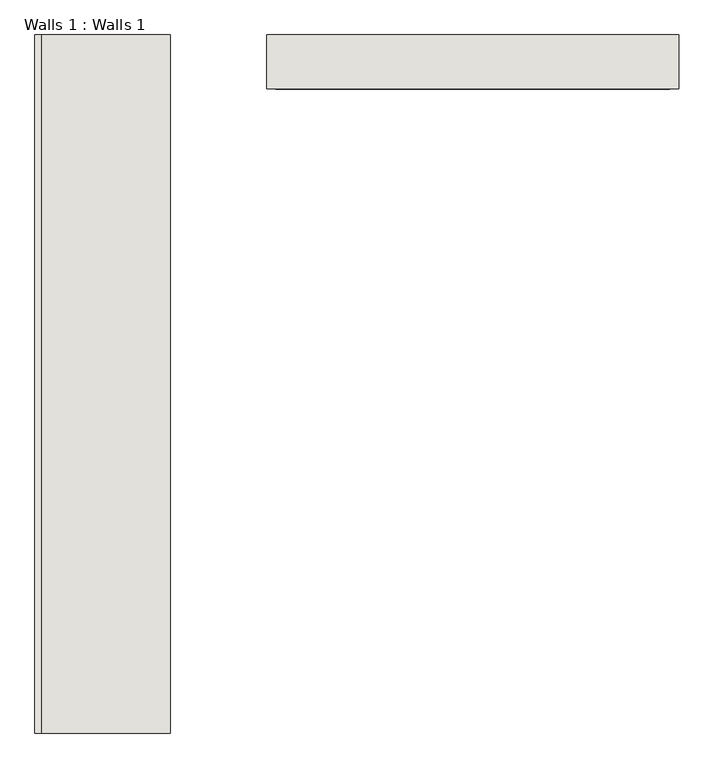
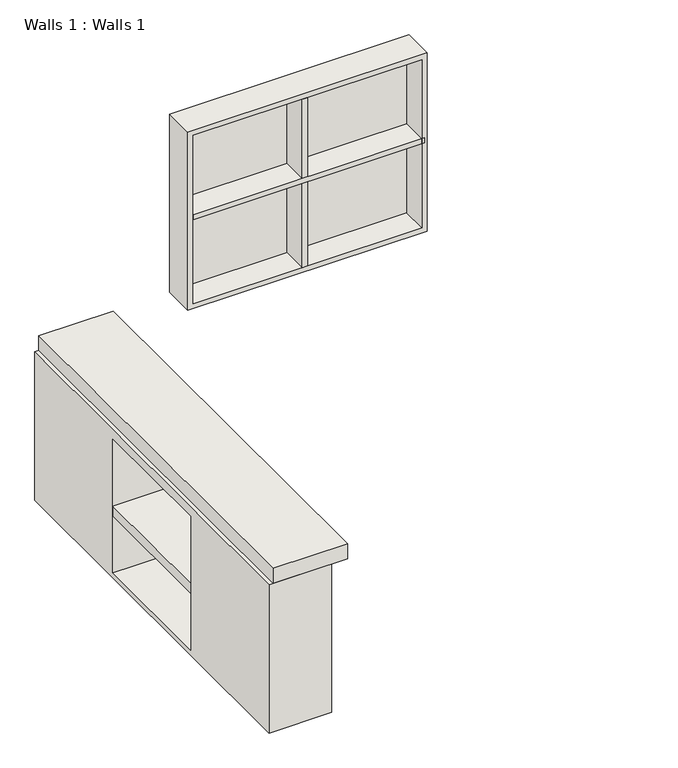
"""IFC4 building model written with IfcOpenShell, lengths in millimetres: wall geometry, Walls 1 : Walls 1."""

from ifc_helpers import new_model, si_unit, frame, origin, place, context, project, spatial, polyline, outline, extrude, faceted_brep, source, transform, mapped, element, save


def walls_1_walls_1_7121089b(model_context):
    return source(origin(), model_context, "Body", "SolidModel", [
        extrude(outline(polyline([(-4669.7681702, -2647.557676), (-4669.7681702, -2774.557676), (-5793.7181702, -2774.557676), (-5793.7181702, -2647.557676), (-4669.7681702, -2647.557676)])), frame((0.0, 0.0, 1322.4031259), z_axis=(0.0, 0.0, 1.0), x_axis=(1.0, 0.0, 0.0)), (0.0, 0.0, 1.0), 25.4),
        extrude(outline(polyline([(-5263.4931702, -2774.557676), (-5263.4931702, -2647.557676), (-5238.0931702, -2647.557676), (-5238.0931702, -2774.557676), (-5263.4931702, -2774.557676)])), frame((0.0, 0.0, 890.6031259), z_axis=(0.0, 0.0, 1.0), x_axis=(1.0, 0.0, 0.0)), (0.0, 0.0, 1.0), 863.6),
        faceted_brep([(-4657.0681702, -2774.557676, 865.2031259), (-4657.0681702, -2774.557676, 1779.6031259), (-5819.1181702, -2774.557676, 1779.6031259), (-5819.1181702, -2774.557676, 865.2031259), (-4682.4681702, -2774.557676, 1754.2031259), (-4682.4681702, -2774.557676, 890.6031259), (-5793.7181702, -2774.557676, 890.6031259), (-5793.7181702, -2774.557676, 1754.2031259), (-4657.0681702, -2622.157676, 865.2031259), (-5819.1181702, -2622.157676, 865.2031259), (-5819.1181702, -2622.157676, 1779.6031259), (-4657.0681702, -2622.157676, 1779.6031259), (-4682.4681702, -2647.557676, 1754.2031259), (-5793.7181702, -2647.557676, 1754.2031259), (-5793.7181702, -2647.557676, 890.6031259), (-4682.4681702, -2647.557676, 890.6031259)], [[[0, 1, 2, 3], [4, 5, 6, 7]], [[8, 9, 10, 11]], [[1, 0, 8, 11]], [[2, 1, 11, 10]], [[3, 2, 10, 9]], [[0, 3, 9, 8]], [[12, 13, 14, 15]], [[12, 15, 5, 4]], [[15, 14, 6, 5]], [[14, 13, 7, 6]], [[13, 12, 4, 7]]]),
        extrude(outline(polyline([(-6454.1181702, -2622.157676), (-6092.1681702, -2622.157676), (-6092.1681702, -4590.657676), (-6454.1181702, -4590.657676), (-6454.1181702, -2622.157676)])), frame((0.0, 0.0, 789.0031259), z_axis=(0.0, 0.0, 1.0), x_axis=(1.0, 0.0, 0.0)), (0.0, 0.0, 1.0), 76.2),
        extrude(outline(polyline([(-6165.8877015, -3282.4431283), (-6165.8877015, -3592.120176), (-6170.9478577, -3592.120176), (-6170.9478577, -3282.4431283), (-6165.8877015, -3282.4431283)])), frame((0.0, 0.0, 45.5519176), z_axis=(0.0, 0.0, 1.0), x_axis=(1.0, 0.0, 0.0)), (0.0, 0.0, 1.0), 685.8),
        extrude(outline(polyline([(-6163.308014, -3603.6829064), (-6163.308014, -3930.257676), (-6168.3681702, -3930.257676), (-6168.3681702, -3603.6829064), (-6163.308014, -3603.6829064)])), frame((0.0, 0.0, 52.4031259), z_axis=(0.0, 0.0, 1.0), x_axis=(1.0, 0.0, 0.0)), (0.0, 0.0, 1.0), 685.8),
        extrude(outline(polyline([(-6168.3681702, -3277.1081367), (-6168.3681702, -3930.257676), (-6473.1681702, -3930.257676), (-6473.1681702, -3277.1081367), (-6168.3681702, -3277.1081367)])), frame((0.0, 0.0, 344.5031259), z_axis=(0.0, 0.0, 1.0), x_axis=(1.0, 0.0, 0.0)), (0.0, 0.0, 1.0), 50.8),
        extrude(outline(polyline([(-2622.157676, 27.0031259), (-4590.657676, 27.0031259), (-4590.657676, 789.0031259), (-2622.157676, 789.0031259), (-2622.157676, 27.0031259)]), holes=[polyline([(-3277.1081367, 52.4031259), (-3277.1081367, 738.2031259), (-3930.257676, 738.2031259), (-3930.257676, 52.4031259), (-3277.1081367, 52.4031259)])]), frame((-6473.1681702, 0.0, 0.0), z_axis=(1.0, 0.0, 0.0), x_axis=(0.0, 1.0, 0.0)), (0.0, 0.0, 1.0), 304.8),
        extrude(outline(polyline([(-6165.7884827, -2647.557676), (-6165.7884827, -3257.157676), (-6168.3681702, -3257.157676), (-6168.3681702, -2647.557676), (-6165.7884827, -2647.557676)])), frame((0.0, 0.0, 55.5781259), z_axis=(0.0, 0.0, 1.0), x_axis=(1.0, 0.0, 0.0)), (0.0, 0.0, 1.0), 298.45),
        extrude(outline(polyline([(-6165.7884827, -2647.557676), (-6165.7884827, -3257.157676), (-6168.3681702, -3257.157676), (-6168.3681702, -2647.557676), (-6165.7884827, -2647.557676)])), frame((0.0, 0.0, 397.8431259), z_axis=(0.0, 0.0, 1.0), x_axis=(1.0, 0.0, 0.0)), (0.0, 0.0, 1.0), 365.76),
        extrude(outline(polyline([(-6165.7884827, -3955.657676), (-6165.7884827, -4565.257676), (-6168.3681702, -4565.257676), (-6168.3681702, -3955.657676), (-6165.7884827, -3955.657676)])), frame((0.0, 0.0, 55.5781259), z_axis=(0.0, 0.0, 1.0), x_axis=(1.0, 0.0, 0.0)), (0.0, 0.0, 1.0), 298.45),
        extrude(outline(polyline([(-6165.7884827, -3955.657676), (-6165.7884827, -4565.257676), (-6168.3681702, -4565.257676), (-6168.3681702, -3955.657676), (-6165.7884827, -3955.657676)])), frame((0.0, 0.0, 397.8431259), z_axis=(0.0, 0.0, 1.0), x_axis=(1.0, 0.0, 0.0)), (0.0, 0.0, 1.0), 365.76),
    ])


if __name__ == "__main__":
    model = new_model("IFC4")
    model_context = context("Model", 3, world=origin())
    ifc_project = project(units=[si_unit("LENGTHUNIT", "METRE", prefix="MILLI")], contexts=[model_context])
    site = spatial("IfcSite", under=ifc_project)
    building = spatial("IfcBuilding", under=site)
    placement = place(None, origin())
    walls_1_walls_1_shape = walls_1_walls_1_7121089b(model_context)
    element("IfcWall", 1, ObjectType="Walls 1 : Walls 1", at=placement, inside=building, context=model_context, shape_type="MappedRepresentation", body=[
        mapped(walls_1_walls_1_shape, transform((0.0, 0.0, 0.0), x_axis=(1.0, 0.0, 0.0), y_axis=(0.0, 1.0, 0.0), z_axis=(0.0, 0.0, 1.0))),
    ])
    save(model, "model.ifc")

# Revit data of these elements
# Element 1 (IfcWall, "Walls 1 : Walls 1")
#   Materials on its faces: "drawers", "wood", "clear glass", "stone", "Default Wall"
# Materials
#   "drawers": class "Generic", colour RGB 121 66 39, transparency 0, Cost = 0
#   "wood": class "Generic", colour RGB 255 226 181, transparency 0, Cost = 0
#   "clear glass": class "Generic", colour RGB 141 181 235, transparency 0.9, Cost = 0
#   "stone": class "Generic", colour RGB 125 126 130, transparency 0, Cost = 0
#   "Default Wall": colour RGB 128 128 128, transparency 0
